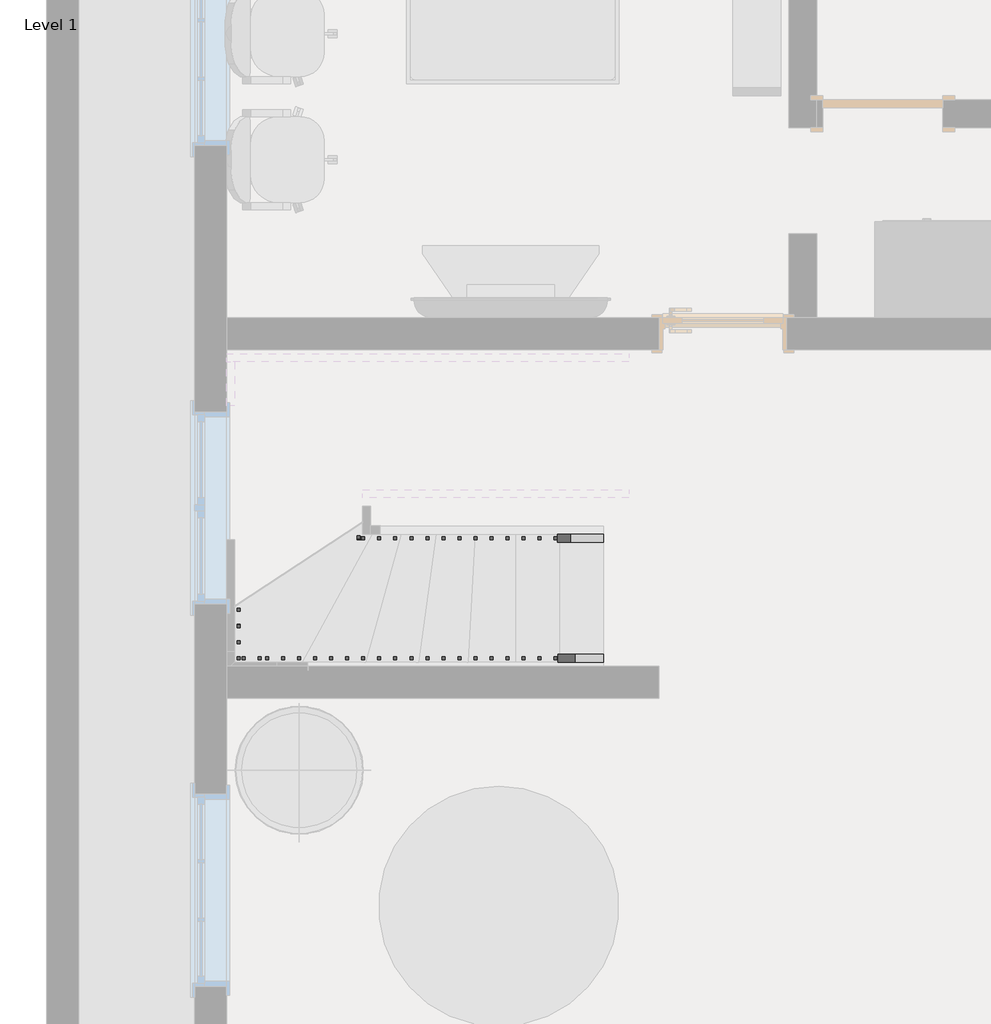
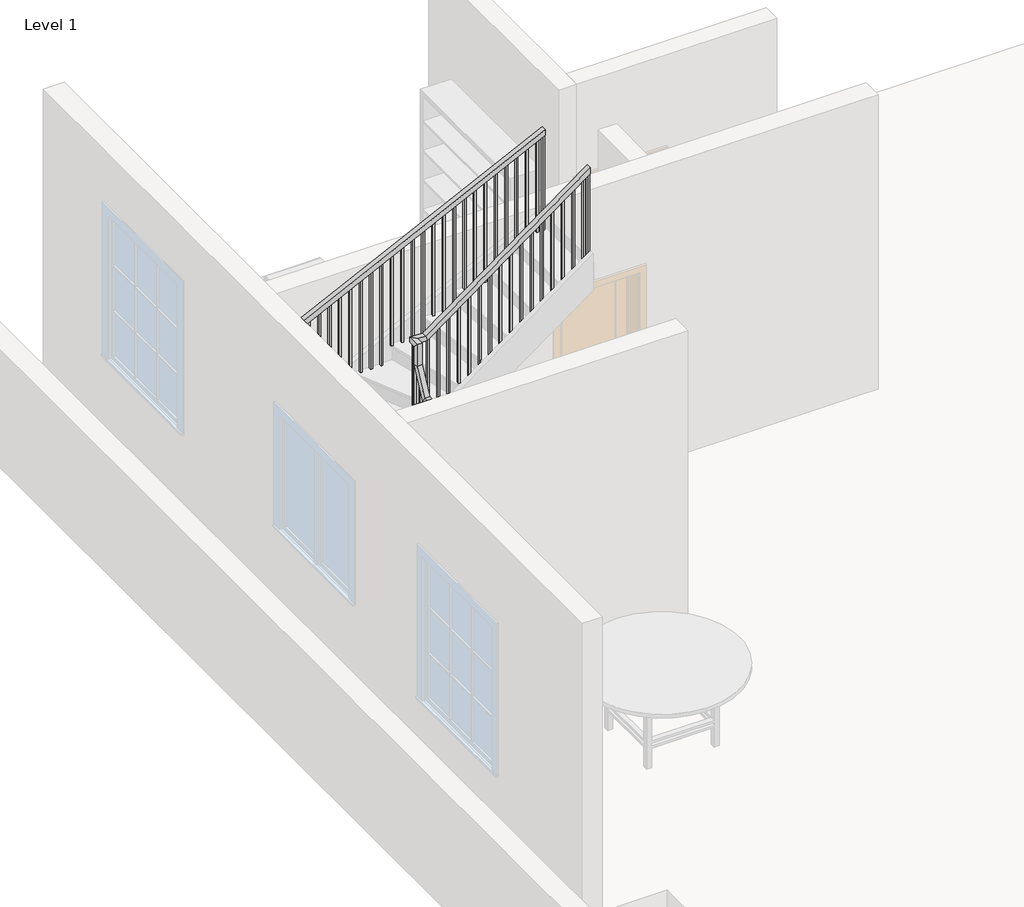
# One storey, part 2 of 3: 2 railings.
"""IFC4 building model written with IfcOpenShell, lengths in millimetres."""

from ifc_helpers import new_model, si_unit, frame, origin, place, context, project, spatial, polyline, outline, extrude, faceted_brep, element, save

model = new_model("IFC4")

# Units and contexts
model_context = context("Model", 3, world=origin())
ifc_project = project(units=[si_unit("LENGTHUNIT", "METRE", prefix="MILLI")], contexts=[model_context])

# Site, building, storey
site = spatial("IfcSite", under=ifc_project)
building = spatial("IfcBuilding", under=site)
storey = spatial("IfcBuildingStorey", under=building, Name="Level 1", Elevation=0.0)

# Railings
placement = place(None, origin())
element("IfcRailing", 1, ObjectType="Handrail - Rectangular", at=placement, inside=storey, context=model_context, shape_type="SolidModel", body=[
    faceted_brep([(-12253.9414615, 8938.3162111, 1054.0374735), (-12253.9414615, 8938.3162111, 991.6664218), (-12253.9414615, 8989.1162111, 991.6664218), (-12253.9414615, 8989.1162111, 1054.0374735), (-13705.4731534, 8938.3162111, 2088.0288176), (-13756.2731534, 8938.3162111, 2061.8448919), (-13756.2731534, 8989.1162111, 2061.8448919), (-13705.4731534, 8989.1162111, 2088.0288176), (-13705.4731534, 8938.3162111, 2341.1218659), (-13756.2731534, 8938.3162111, 2290.3218659), (-13756.2731534, 8989.1162111, 2290.3218659), (-13705.4731534, 8989.1162111, 2341.1218659), (-13832.4731534, 8938.3162111, 2341.1218659), (-13832.4731534, 8938.3162111, 2290.3218659), (-13781.6731534, 8989.1162111, 2290.3218659), (-13781.6731534, 8989.1162111, 2341.1218659), (-13832.4731534, 9065.3162111, 2341.1218659), (-13832.4731534, 9096.7018628, 2290.3218659), (-13781.6731534, 9096.7018628, 2290.3218659), (-13781.6731534, 9065.3162111, 2341.1218659), (-13832.4731534, 9192.3162111, 2594.9324677), (-13832.4731534, 9243.1162111, 2582.9322113), (-13781.6731534, 9243.1162111, 2582.9322113), (-13781.6731534, 9192.3162111, 2594.9324677), (-13832.4731534, 9192.3162111, 2819.759768), (-13832.4731534, 9243.1162111, 2768.959768), (-13781.6731534, 9243.1162111, 2768.959768), (-13781.6731534, 9192.3162111, 2819.759768), (-13832.4731534, 9319.3162111, 2819.759768), (-13832.4731534, 9319.3162111, 2768.959768), (-13781.6731534, 9268.5162111, 2768.959768), (-13781.6731534, 9268.5162111, 2819.759768), (-13705.4731534, 9319.3162111, 2819.759768), (-13688.9113924, 9319.3162111, 2768.959768), (-13688.9113924, 9268.5162111, 2768.959768), (-13705.4731534, 9268.5162111, 2819.759768), (-12092.016007, 9319.3162111, 3996.9124676), (-12092.016007, 9268.5162111, 3996.9124676), (-12092.016007, 9268.5162111, 3934.0292699), (-12092.016007, 9319.3162111, 3934.0292699)], [[[0, 1, 2, 3]], [[1, 0, 4, 5]], [[2, 1, 5, 6]], [[3, 2, 6, 7]], [[0, 3, 7, 4]], [[5, 4, 8, 9]], [[6, 5, 9, 10]], [[7, 6, 10, 11]], [[4, 7, 11, 8]], [[9, 8, 12, 13]], [[10, 9, 13, 14]], [[11, 10, 14, 15]], [[8, 11, 15, 12]], [[13, 12, 16, 17]], [[14, 13, 17, 18]], [[15, 14, 18, 19]], [[12, 15, 19, 16]], [[17, 16, 20, 21]], [[18, 17, 21, 22]], [[19, 18, 22, 23]], [[16, 19, 23, 20]], [[21, 20, 24, 25]], [[22, 21, 25, 26]], [[23, 22, 26, 27]], [[20, 23, 27, 24]], [[25, 24, 28, 29]], [[26, 25, 29, 30]], [[27, 26, 30, 31]], [[24, 27, 31, 28]], [[29, 28, 32, 33]], [[30, 29, 33, 34]], [[31, 30, 34, 35]], [[28, 31, 35, 32]], [[36, 37, 38, 39]], [[33, 32, 36, 39]], [[34, 33, 39, 38]], [[35, 34, 38, 37]], [[32, 35, 37, 36]]]),
    extrude(outline(polyline([(3901.8855094, -12136.0736558), (3887.986932, -12155.1236558), (2878.6666667, -12155.1236558), (2878.6666667, -12136.0736558), (3901.8855094, -12136.0736558)])), frame((0.0, 9284.3912111, 0.0), z_axis=(0.0, 1.0, 0.0), x_axis=(0.0, 0.0, 1.0)), (0.0, 0.0, 1.0), 19.05),
    extrude(outline(polyline([(3827.7597636, -12237.6736558), (3813.8611863, -12256.7236558), (2878.6666667, -12256.7236558), (2878.6666667, -12237.6736558), (3827.7597636, -12237.6736558)])), frame((0.0, 9284.3912111, 0.0), z_axis=(0.0, 1.0, 0.0), x_axis=(0.0, 0.0, 1.0)), (0.0, 0.0, 1.0), 19.05),
    extrude(outline(polyline([(3753.6340178, -12339.2736558), (3739.7354405, -12358.3236558), (2878.6666667, -12358.3236558), (2878.6666667, -12339.2736558), (3753.6340178, -12339.2736558)])), frame((0.0, 9284.3912111, 0.0), z_axis=(0.0, 1.0, 0.0), x_axis=(0.0, 0.0, 1.0)), (0.0, 0.0, 1.0), 19.05),
    extrude(outline(polyline([(3679.508272, -12440.8736558), (3665.6096947, -12459.9236558), (2709.3333333, -12459.9236558), (2709.3333333, -12440.8736558), (3679.508272, -12440.8736558)])), frame((0.0, 9284.3912111, 0.0), z_axis=(0.0, 1.0, 0.0), x_axis=(0.0, 0.0, 1.0)), (0.0, 0.0, 1.0), 19.05),
    extrude(outline(polyline([(3605.3825262, -12542.4736558), (3591.4839489, -12561.5236558), (2709.3333333, -12561.5236558), (2709.3333333, -12542.4736558), (3605.3825262, -12542.4736558)])), frame((0.0, 9284.3912111, 0.0), z_axis=(0.0, 1.0, 0.0), x_axis=(0.0, 0.0, 1.0)), (0.0, 0.0, 1.0), 19.05),
    extrude(outline(polyline([(3531.2567804, -12644.0736558), (3517.3582031, -12663.1236558), (2540.0, -12663.1236558), (2540.0, -12644.0736558), (3531.2567804, -12644.0736558)])), frame((0.0, 9284.3912111, 0.0), z_axis=(0.0, 1.0, 0.0), x_axis=(0.0, 0.0, 1.0)), (0.0, 0.0, 1.0), 19.05),
    extrude(outline(polyline([(3457.1310346, -12745.6736558), (3443.2324573, -12764.7236558), (2540.0, -12764.7236558), (2540.0, -12745.6736558), (3457.1310346, -12745.6736558)])), frame((0.0, 9284.3912111, 0.0), z_axis=(0.0, 1.0, 0.0), x_axis=(0.0, 0.0, 1.0)), (0.0, 0.0, 1.0), 19.05),
    extrude(outline(polyline([(3383.0052889, -12847.2736558), (3369.1067115, -12866.3236558), (2540.0, -12866.3236558), (2540.0, -12847.2736558), (3383.0052889, -12847.2736558)])), frame((0.0, 9284.3912111, 0.0), z_axis=(0.0, 1.0, 0.0), x_axis=(0.0, 0.0, 1.0)), (0.0, 0.0, 1.0), 19.05),
    extrude(outline(polyline([(3308.8795431, -12948.8736558), (3294.9809657, -12967.9236558), (2370.6666667, -12967.9236558), (2370.6666667, -12948.8736558), (3308.8795431, -12948.8736558)])), frame((0.0, 9284.3912111, 0.0), z_axis=(0.0, 1.0, 0.0), x_axis=(0.0, 0.0, 1.0)), (0.0, 0.0, 1.0), 19.05),
    extrude(outline(polyline([(3234.7537973, -13050.4736558), (3220.8552199, -13069.5236558), (2370.6666667, -13069.5236558), (2370.6666667, -13050.4736558), (3234.7537973, -13050.4736558)])), frame((0.0, 9284.3912111, 0.0), z_axis=(0.0, 1.0, 0.0), x_axis=(0.0, 0.0, 1.0)), (0.0, 0.0, 1.0), 19.05),
    extrude(outline(polyline([(3160.6280515, -13152.0736558), (3146.7294741, -13171.1236558), (2201.3333333, -13171.1236558), (2201.3333333, -13152.0736558), (3160.6280515, -13152.0736558)])), frame((0.0, 9284.3912111, 0.0), z_axis=(0.0, 1.0, 0.0), x_axis=(0.0, 0.0, 1.0)), (0.0, 0.0, 1.0), 19.05),
    extrude(outline(polyline([(3086.5023057, -13253.6736558), (3072.6037284, -13272.7236558), (2201.3333333, -13272.7236558), (2201.3333333, -13253.6736558), (3086.5023057, -13253.6736558)])), frame((0.0, 9284.3912111, 0.0), z_axis=(0.0, 1.0, 0.0), x_axis=(0.0, 0.0, 1.0)), (0.0, 0.0, 1.0), 19.05),
    extrude(outline(polyline([(3012.3765599, -13355.2736558), (2998.4779826, -13374.3236558), (2201.3333333, -13374.3236558), (2201.3333333, -13355.2736558), (3012.3765599, -13355.2736558)])), frame((0.0, 9284.3912111, 0.0), z_axis=(0.0, 1.0, 0.0), x_axis=(0.0, 0.0, 1.0)), (0.0, 0.0, 1.0), 19.05),
    extrude(outline(polyline([(2938.2508141, -13456.8736558), (2924.3522368, -13475.9236558), (2032.0, -13475.9236558), (2032.0, -13456.8736558), (2938.2508141, -13456.8736558)])), frame((0.0, 9284.3912111, 0.0), z_axis=(0.0, 1.0, 0.0), x_axis=(0.0, 0.0, 1.0)), (0.0, 0.0, 1.0), 19.05),
    extrude(outline(polyline([(2864.1250683, -13558.4736558), (2850.226491, -13577.5236558), (2032.0, -13577.5236558), (2032.0, -13558.4736558), (2864.1250683, -13558.4736558)])), frame((0.0, 9284.3912111, 0.0), z_axis=(0.0, 1.0, 0.0), x_axis=(0.0, 0.0, 1.0)), (0.0, 0.0, 1.0), 19.05),
    extrude(outline(polyline([(2789.9993225, -13660.0736558), (2776.1007452, -13679.1236558), (1862.6666667, -13679.1236558), (1862.6666667, -13660.0736558), (2789.9993225, -13660.0736558)])), frame((0.0, 9284.3912111, 0.0), z_axis=(0.0, 1.0, 0.0), x_axis=(0.0, 0.0, 1.0)), (0.0, 0.0, 1.0), 19.05),
    extrude(outline(polyline([(-13797.5481534, 9264.5777982), (-13816.5981534, 9264.5777982), (-13816.5981534, 9283.6277982), (-13797.5481534, 9283.6277982), (-13797.5481534, 9264.5777982)])), frame((0.0, 0.0, 1693.3333333), z_axis=(0.0, 0.0, 1.0), x_axis=(1.0, 0.0, 0.0)), (0.0, 0.0, 1.0), 1075.6264347),
    extrude(outline(polyline([(9162.9777982, 2422.7748977), (9182.0277982, 2460.846488), (9182.0277982, 1524.0), (9162.9777982, 1524.0), (9162.9777982, 2422.7748977)])), frame((-13816.5981534, 0.0, 0.0), z_axis=(1.0, 0.0, 0.0), x_axis=(0.0, 1.0, 0.0)), (0.0, 0.0, 1.0), 19.05),
    extrude(outline(polyline([(9061.3777982, 2219.7264162), (9080.4277982, 2257.7980065), (9080.4277982, 1354.6666667), (9061.3777982, 1354.6666667), (9061.3777982, 2219.7264162)])), frame((-13816.5981534, 0.0, 0.0), z_axis=(1.0, 0.0, 0.0), x_axis=(0.0, 1.0, 0.0)), (0.0, 0.0, 1.0), 19.05),
    extrude(outline(polyline([(-13768.4164615, 8973.2412111), (-13768.4164615, 8954.1912111), (-13787.4664615, 8954.1912111), (-13787.4664615, 8973.2412111), (-13768.4164615, 8973.2412111)])), frame((0.0, 0.0, 1185.3333333), z_axis=(0.0, 0.0, 1.0), x_axis=(1.0, 0.0, 0.0)), (0.0, 0.0, 1.0), 1104.9885325),
    extrude(outline(polyline([(1998.1208647, -13666.8164615), (2011.691037, -13685.8664615), (1016.0, -13685.8664615), (1016.0, -13666.8164615), (1998.1208647, -13666.8164615)])), frame((0.0, 8954.1912111, 0.0), z_axis=(0.0, 1.0, 0.0), x_axis=(0.0, 0.0, 1.0)), (0.0, 0.0, 1.0), 19.05),
    extrude(outline(polyline([(1925.7466126, -13565.2164615), (1939.3167849, -13584.2664615), (1016.0, -13584.2664615), (1016.0, -13565.2164615), (1925.7466126, -13565.2164615)])), frame((0.0, 8954.1912111, 0.0), z_axis=(0.0, 1.0, 0.0), x_axis=(0.0, 0.0, 1.0)), (0.0, 0.0, 1.0), 19.05),
    extrude(outline(polyline([(1853.3723605, -13463.6164615), (1866.9425328, -13482.6664615), (846.6666667, -13482.6664615), (846.6666667, -13463.6164615), (1853.3723605, -13463.6164615)])), frame((0.0, 8954.1912111, 0.0), z_axis=(0.0, 1.0, 0.0), x_axis=(0.0, 0.0, 1.0)), (0.0, 0.0, 1.0), 19.05),
    extrude(outline(polyline([(1780.9981085, -13362.0164615), (1794.5682807, -13381.0664615), (846.6666667, -13381.0664615), (846.6666667, -13362.0164615), (1780.9981085, -13362.0164615)])), frame((0.0, 8954.1912111, 0.0), z_axis=(0.0, 1.0, 0.0), x_axis=(0.0, 0.0, 1.0)), (0.0, 0.0, 1.0), 19.05),
    extrude(outline(polyline([(1708.6238564, -13260.4164615), (1722.1940286, -13279.4664615), (677.3333333, -13279.4664615), (677.3333333, -13260.4164615), (1708.6238564, -13260.4164615)])), frame((0.0, 8954.1912111, 0.0), z_axis=(0.0, 1.0, 0.0), x_axis=(0.0, 0.0, 1.0)), (0.0, 0.0, 1.0), 19.05),
    extrude(outline(polyline([(1636.2496043, -13158.8164615), (1649.8197766, -13177.8664615), (677.3333333, -13177.8664615), (677.3333333, -13158.8164615), (1636.2496043, -13158.8164615)])), frame((0.0, 8954.1912111, 0.0), z_axis=(0.0, 1.0, 0.0), x_axis=(0.0, 0.0, 1.0)), (0.0, 0.0, 1.0), 19.05),
    extrude(outline(polyline([(1563.8753522, -13057.2164615), (1577.4455245, -13076.2664615), (508.0, -13076.2664615), (508.0, -13057.2164615), (1563.8753522, -13057.2164615)])), frame((0.0, 8954.1912111, 0.0), z_axis=(0.0, 1.0, 0.0), x_axis=(0.0, 0.0, 1.0)), (0.0, 0.0, 1.0), 19.05),
    extrude(outline(polyline([(1491.5011002, -12955.6164615), (1505.0712724, -12974.6664615), (508.0, -12974.6664615), (508.0, -12955.6164615), (1491.5011002, -12955.6164615)])), frame((0.0, 8954.1912111, 0.0), z_axis=(0.0, 1.0, 0.0), x_axis=(0.0, 0.0, 1.0)), (0.0, 0.0, 1.0), 19.05),
    extrude(outline(polyline([(1419.1268481, -12854.0164615), (1432.6970203, -12873.0664615), (508.0, -12873.0664615), (508.0, -12854.0164615), (1419.1268481, -12854.0164615)])), frame((0.0, 8954.1912111, 0.0), z_axis=(0.0, 1.0, 0.0), x_axis=(0.0, 0.0, 1.0)), (0.0, 0.0, 1.0), 19.05),
    extrude(outline(polyline([(1346.752596, -12752.4164615), (1360.3227683, -12771.4664615), (338.6666667, -12771.4664615), (338.6666667, -12752.4164615), (1346.752596, -12752.4164615)])), frame((0.0, 8954.1912111, 0.0), z_axis=(0.0, 1.0, 0.0), x_axis=(0.0, 0.0, 1.0)), (0.0, 0.0, 1.0), 19.05),
    extrude(outline(polyline([(1274.3783439, -12650.8164615), (1287.9485162, -12669.8664615), (338.6666667, -12669.8664615), (338.6666667, -12650.8164615), (1274.3783439, -12650.8164615)])), frame((0.0, 8954.1912111, 0.0), z_axis=(0.0, 1.0, 0.0), x_axis=(0.0, 0.0, 1.0)), (0.0, 0.0, 1.0), 19.05),
    extrude(outline(polyline([(1202.0040918, -12549.2164615), (1215.5742641, -12568.2664615), (338.6666667, -12568.2664615), (338.6666667, -12549.2164615), (1202.0040918, -12549.2164615)])), frame((0.0, 8954.1912111, 0.0), z_axis=(0.0, 1.0, 0.0), x_axis=(0.0, 0.0, 1.0)), (0.0, 0.0, 1.0), 19.05),
    extrude(outline(polyline([(1129.6298398, -12447.6164615), (1143.200012, -12466.6664615), (169.3333333, -12466.6664615), (169.3333333, -12447.6164615), (1129.6298398, -12447.6164615)])), frame((0.0, 8954.1912111, 0.0), z_axis=(0.0, 1.0, 0.0), x_axis=(0.0, 0.0, 1.0)), (0.0, 0.0, 1.0), 19.05),
    extrude(outline(polyline([(1057.2555877, -12346.0164615), (1070.82576, -12365.0664615), (169.3333333, -12365.0664615), (169.3333333, -12346.0164615), (1057.2555877, -12346.0164615)])), frame((0.0, 8954.1912111, 0.0), z_axis=(0.0, 1.0, 0.0), x_axis=(0.0, 0.0, 1.0)), (0.0, 0.0, 1.0), 19.05),
    extrude(outline(polyline([(-13780.7236558, 9284.3912111), (-13780.7236558, 9303.4412111), (-13761.6736558, 9303.4412111), (-13761.6736558, 9284.3912111), (-13780.7236558, 9284.3912111)])), frame((0.0, 0.0, 1862.6666667), z_axis=(0.0, 0.0, 1.0), x_axis=(1.0, 0.0, 0.0)), (0.0, 0.0, 1.0), 906.2931014),
    extrude(outline(polyline([(-13797.5481534, 9284.3912111), (-13816.5981534, 9284.3912111), (-13816.5981534, 9303.4412111), (-13797.5481534, 9303.4412111), (-13797.5481534, 9284.3912111)])), frame((0.0, 0.0, 1693.3333333), z_axis=(0.0, 0.0, 1.0), x_axis=(1.0, 0.0, 0.0)), (0.0, 0.0, 1.0), 1075.6264347),
    extrude(outline(polyline([(-13797.5481534, 9271.2947138), (-13816.5981534, 9271.2947138), (-13816.5981534, 9290.3447138), (-13797.5481534, 9290.3447138), (-13797.5481534, 9271.2947138)])), frame((0.0, 0.0, 1693.3333333), z_axis=(0.0, 0.0, 1.0), x_axis=(1.0, 0.0, 0.0)), (0.0, 0.0, 1.0), 1075.6264347),
    extrude(outline(polyline([(-13797.5481534, 8959.7777982), (-13816.5981534, 8959.7777982), (-13816.5981534, 8978.8277982), (-13797.5481534, 8978.8277982), (-13797.5481534, 8959.7777982)])), frame((0.0, 0.0, 1185.3333333), z_axis=(0.0, 0.0, 1.0), x_axis=(1.0, 0.0, 0.0)), (0.0, 0.0, 1.0), 1104.9885325),
    extrude(outline(polyline([(-13797.5481534, 8973.2412111), (-13797.5481534, 8954.1912111), (-13816.5981534, 8954.1912111), (-13816.5981534, 8973.2412111), (-13797.5481534, 8973.2412111)])), frame((0.0, 0.0, 1185.3333333), z_axis=(0.0, 0.0, 1.0), x_axis=(1.0, 0.0, 0.0)), (0.0, 0.0, 1.0), 1104.9885325),
    extrude(outline(polyline([(-13781.8747892, 8973.2412111), (-13781.8747892, 8954.1912111), (-13800.9247892, 8954.1912111), (-13800.9247892, 8973.2412111), (-13781.8747892, 8973.2412111)])), frame((0.0, 0.0, 1185.3333333), z_axis=(0.0, 0.0, 1.0), x_axis=(1.0, 0.0, 0.0)), (0.0, 0.0, 1.0), 1104.9885325),
    extrude(outline(polyline([(3934.0292699, -12092.016007), (3920.1306926, -12111.066007), (2878.6666667, -12111.066007), (2878.6666667, -12092.016007), (3934.0292699, -12092.016007)])), frame((0.0, 9284.3912111, 0.0), z_axis=(0.0, 1.0, 0.0), x_axis=(0.0, 0.0, 1.0)), (0.0, 0.0, 1.0), 19.05),
    extrude(outline(polyline([(991.6664218, -12253.9414615), (1005.236594, -12272.9914615), (169.3333333, -12272.9914615), (169.3333333, -12253.9414615), (991.6664218, -12253.9414615)])), frame((0.0, 8954.1912111, 0.0), z_axis=(0.0, 1.0, 0.0), x_axis=(0.0, 0.0, 1.0)), (0.0, 0.0, 1.0), 19.05),
])
element("IfcRailing", 2, ObjectType="Handrail - Rectangular", at=placement, inside=storey, context=model_context, shape_type="SolidModel", body=[
    faceted_brep([(-12253.9414615, 8176.3162111, 1108.1974031), (-12253.9414615, 8176.3162111, 1050.9747805), (-12253.9414615, 8227.1162111, 1050.9747805), (-12253.9414615, 8227.1162111, 1108.1974031), (-14435.851857, 8176.3162111, 2239.520782), (-14448.2387549, 8176.3162111, 2188.720782), (-14448.2387549, 8227.1162111, 2188.720782), (-14435.851857, 8227.1162111, 2239.520782), (-14594.4731534, 8176.3162111, 2239.520782), (-14594.4731534, 8176.3162111, 2188.720782), (-14543.6731534, 8227.1162111, 2188.720782), (-14543.6731534, 8227.1162111, 2239.520782), (-14594.4731534, 8407.7273211, 2239.520782), (-14594.4731534, 8416.0171351, 2188.720782), (-14543.6731534, 8416.0171351, 2188.720782), (-14543.6731534, 8407.7273211, 2239.520782), (-14594.4731534, 9947.9383629, 2755.9527245), (-14594.4731534, 9956.2281769, 2705.1527245), (-14543.6731534, 9956.2281769, 2705.1527245), (-14543.6731534, 9947.9383629, 2755.9527245), (-14594.4731534, 10081.3162111, 2755.9527245), (-14594.4731534, 10081.3162111, 2705.1527245), (-14543.6731534, 10030.5162111, 2705.1527245), (-14543.6731534, 10030.5162111, 2755.9527245), (-14494.942349, 10081.3162111, 2755.9527245), (-14483.1999894, 10081.3162111, 2705.1527245), (-14483.1999894, 10030.5162111, 2705.1527245), (-14494.942349, 10030.5162111, 2755.9527245), (-12092.016007, 10081.3162111, 3929.523479), (-12092.016007, 10030.5162111, 3929.523479), (-12092.016007, 10030.5162111, 3872.9886008), (-12092.016007, 10081.3162111, 3872.9886008)], [[[0, 1, 2, 3]], [[1, 0, 4, 5]], [[2, 1, 5, 6]], [[3, 2, 6, 7]], [[0, 3, 7, 4]], [[5, 4, 8, 9]], [[6, 5, 9, 10]], [[7, 6, 10, 11]], [[4, 7, 11, 8]], [[9, 8, 12, 13]], [[10, 9, 13, 14]], [[11, 10, 14, 15]], [[8, 11, 15, 12]], [[13, 12, 16, 17]], [[14, 13, 17, 18]], [[15, 14, 18, 19]], [[12, 15, 19, 16]], [[17, 16, 20, 21]], [[18, 17, 21, 22]], [[19, 18, 22, 23]], [[16, 19, 23, 20]], [[21, 20, 24, 25]], [[22, 21, 25, 26]], [[23, 22, 26, 27]], [[20, 23, 27, 24]], [[28, 29, 30, 31]], [[25, 24, 28, 31]], [[26, 25, 31, 30]], [[27, 26, 30, 29]], [[24, 27, 29, 28]]]),
    extrude(outline(polyline([(3836.0410669, -12167.667349), (2878.6666667, -12167.667349), (2878.6666667, -12148.617349), (3845.3449404, -12148.617349), (3836.0410669, -12167.667349)])), frame((0.0, 10046.3912111, 0.0), z_axis=(0.0, 1.0, 0.0), x_axis=(0.0, 0.0, 1.0)), (0.0, 0.0, 1.0), 19.05),
    extrude(outline(polyline([(3786.4204079, -12269.267349), (2878.6666667, -12269.267349), (2878.6666667, -12250.217349), (3795.7242814, -12250.217349), (3786.4204079, -12269.267349)])), frame((0.0, 10046.3912111, 0.0), z_axis=(0.0, 1.0, 0.0), x_axis=(0.0, 0.0, 1.0)), (0.0, 0.0, 1.0), 19.05),
    extrude(outline(polyline([(3736.7997488, -12370.867349), (2878.6666667, -12370.867349), (2878.6666667, -12351.817349), (3746.1036224, -12351.817349), (3736.7997488, -12370.867349)])), frame((0.0, 10046.3912111, 0.0), z_axis=(0.0, 1.0, 0.0), x_axis=(0.0, 0.0, 1.0)), (0.0, 0.0, 1.0), 19.05),
    extrude(outline(polyline([(3687.1790898, -12472.467349), (2709.3333333, -12472.467349), (2709.3333333, -12453.417349), (3696.4829634, -12453.417349), (3687.1790898, -12472.467349)])), frame((0.0, 10046.3912111, 0.0), z_axis=(0.0, 1.0, 0.0), x_axis=(0.0, 0.0, 1.0)), (0.0, 0.0, 1.0), 19.05),
    extrude(outline(polyline([(3637.5584308, -12574.067349), (2709.3333333, -12574.067349), (2709.3333333, -12555.017349), (3646.8623044, -12555.017349), (3637.5584308, -12574.067349)])), frame((0.0, 10046.3912111, 0.0), z_axis=(0.0, 1.0, 0.0), x_axis=(0.0, 0.0, 1.0)), (0.0, 0.0, 1.0), 19.05),
    extrude(outline(polyline([(3587.9377718, -12675.667349), (2540.0, -12675.667349), (2540.0, -12656.617349), (3597.2416454, -12656.617349), (3587.9377718, -12675.667349)])), frame((0.0, 10046.3912111, 0.0), z_axis=(0.0, 1.0, 0.0), x_axis=(0.0, 0.0, 1.0)), (0.0, 0.0, 1.0), 19.05),
    extrude(outline(polyline([(3538.3171128, -12777.267349), (2540.0, -12777.267349), (2540.0, -12758.217349), (3547.6209864, -12758.217349), (3538.3171128, -12777.267349)])), frame((0.0, 10046.3912111, 0.0), z_axis=(0.0, 1.0, 0.0), x_axis=(0.0, 0.0, 1.0)), (0.0, 0.0, 1.0), 19.05),
    extrude(outline(polyline([(3488.6964538, -12878.867349), (2540.0, -12878.867349), (2540.0, -12859.817349), (3498.0003273, -12859.817349), (3488.6964538, -12878.867349)])), frame((0.0, 10046.3912111, 0.0), z_axis=(0.0, 1.0, 0.0), x_axis=(0.0, 0.0, 1.0)), (0.0, 0.0, 1.0), 19.05),
    extrude(outline(polyline([(3439.0757948, -12980.467349), (2370.6666667, -12980.467349), (2370.6666667, -12961.417349), (3448.3796683, -12961.417349), (3439.0757948, -12980.467349)])), frame((0.0, 10046.3912111, 0.0), z_axis=(0.0, 1.0, 0.0), x_axis=(0.0, 0.0, 1.0)), (0.0, 0.0, 1.0), 19.05),
    extrude(outline(polyline([(3389.4551357, -13082.067349), (2370.6666667, -13082.067349), (2370.6666667, -13063.017349), (3398.7590093, -13063.017349), (3389.4551357, -13082.067349)])), frame((0.0, 10046.3912111, 0.0), z_axis=(0.0, 1.0, 0.0), x_axis=(0.0, 0.0, 1.0)), (0.0, 0.0, 1.0), 19.05),
    extrude(outline(polyline([(3339.8344767, -13183.667349), (2370.6666667, -13183.667349), (2370.6666667, -13164.617349), (3349.1383503, -13164.617349), (3339.8344767, -13183.667349)])), frame((0.0, 10046.3912111, 0.0), z_axis=(0.0, 1.0, 0.0), x_axis=(0.0, 0.0, 1.0)), (0.0, 0.0, 1.0), 19.05),
    extrude(outline(polyline([(3290.2138177, -13285.267349), (2201.3333333, -13285.267349), (2201.3333333, -13266.217349), (3299.5176913, -13266.217349), (3290.2138177, -13285.267349)])), frame((0.0, 10046.3912111, 0.0), z_axis=(0.0, 1.0, 0.0), x_axis=(0.0, 0.0, 1.0)), (0.0, 0.0, 1.0), 19.05),
    extrude(outline(polyline([(3240.5931587, -13386.867349), (2201.3333333, -13386.867349), (2201.3333333, -13367.817349), (3249.8970323, -13367.817349), (3240.5931587, -13386.867349)])), frame((0.0, 10046.3912111, 0.0), z_axis=(0.0, 1.0, 0.0), x_axis=(0.0, 0.0, 1.0)), (0.0, 0.0, 1.0), 19.05),
    extrude(outline(polyline([(3190.9724997, -13488.467349), (2201.3333333, -13488.467349), (2201.3333333, -13469.417349), (3200.2763733, -13469.417349), (3190.9724997, -13488.467349)])), frame((0.0, 10046.3912111, 0.0), z_axis=(0.0, 1.0, 0.0), x_axis=(0.0, 0.0, 1.0)), (0.0, 0.0, 1.0), 19.05),
    extrude(outline(polyline([(3141.3518407, -13590.067349), (2201.3333333, -13590.067349), (2201.3333333, -13571.017349), (3150.6557142, -13571.017349), (3141.3518407, -13590.067349)])), frame((0.0, 10046.3912111, 0.0), z_axis=(0.0, 1.0, 0.0), x_axis=(0.0, 0.0, 1.0)), (0.0, 0.0, 1.0), 19.05),
    extrude(outline(polyline([(3091.7311817, -13691.667349), (2032.0, -13691.667349), (2032.0, -13672.617349), (3101.0350552, -13672.617349), (3091.7311817, -13691.667349)])), frame((0.0, 10046.3912111, 0.0), z_axis=(0.0, 1.0, 0.0), x_axis=(0.0, 0.0, 1.0)), (0.0, 0.0, 1.0), 19.05),
    extrude(outline(polyline([(3042.1105226, -13793.267349), (2032.0, -13793.267349), (2032.0, -13774.217349), (3051.4143962, -13774.217349), (3042.1105226, -13793.267349)])), frame((0.0, 10046.3912111, 0.0), z_axis=(0.0, 1.0, 0.0), x_axis=(0.0, 0.0, 1.0)), (0.0, 0.0, 1.0), 19.05),
    extrude(outline(polyline([(2992.4898636, -13894.867349), (2032.0, -13894.867349), (2032.0, -13875.817349), (3001.7937372, -13875.817349), (2992.4898636, -13894.867349)])), frame((0.0, 10046.3912111, 0.0), z_axis=(0.0, 1.0, 0.0), x_axis=(0.0, 0.0, 1.0)), (0.0, 0.0, 1.0), 19.05),
    extrude(outline(polyline([(2942.8692046, -13996.467349), (1862.6666667, -13996.467349), (1862.6666667, -13977.417349), (2952.1730782, -13977.417349), (2942.8692046, -13996.467349)])), frame((0.0, 10046.3912111, 0.0), z_axis=(0.0, 1.0, 0.0), x_axis=(0.0, 0.0, 1.0)), (0.0, 0.0, 1.0), 19.05),
    extrude(outline(polyline([(2893.2485456, -14098.067349), (1862.6666667, -14098.067349), (1862.6666667, -14079.017349), (2902.5524192, -14079.017349), (2893.2485456, -14098.067349)])), frame((0.0, 10046.3912111, 0.0), z_axis=(0.0, 1.0, 0.0), x_axis=(0.0, 0.0, 1.0)), (0.0, 0.0, 1.0), 19.05),
    extrude(outline(polyline([(2843.6278866, -14199.667349), (1862.6666667, -14199.667349), (1862.6666667, -14180.617349), (2852.9317602, -14180.617349), (2843.6278866, -14199.667349)])), frame((0.0, 10046.3912111, 0.0), z_axis=(0.0, 1.0, 0.0), x_axis=(0.0, 0.0, 1.0)), (0.0, 0.0, 1.0), 19.05),
    extrude(outline(polyline([(2794.0072276, -14301.267349), (1862.6666667, -14301.267349), (1862.6666667, -14282.217349), (2803.3111011, -14282.217349), (2794.0072276, -14301.267349)])), frame((0.0, 10046.3912111, 0.0), z_axis=(0.0, 1.0, 0.0), x_axis=(0.0, 0.0, 1.0)), (0.0, 0.0, 1.0), 19.05),
    extrude(outline(polyline([(2744.3865686, -14402.867349), (1862.6666667, -14402.867349), (1862.6666667, -14383.817349), (2753.6904421, -14383.817349), (2744.3865686, -14402.867349)])), frame((0.0, 10046.3912111, 0.0), z_axis=(0.0, 1.0, 0.0), x_axis=(0.0, 0.0, 1.0)), (0.0, 0.0, 1.0), 19.05),
    extrude(outline(polyline([(-14578.5981534, 10040.0133629), (-14578.5981534, 10059.0633629), (-14559.5481534, 10059.0633629), (-14559.5481534, 10040.0133629), (-14578.5981534, 10040.0133629)])), frame((0.0, 0.0, 1693.3333333), z_axis=(0.0, 0.0, 1.0), x_axis=(1.0, 0.0, 0.0)), (0.0, 0.0, 1.0), 1011.8193912),
    extrude(outline(polyline([(9941.2523211, 2700.131328), (9941.2523211, 1693.3333333), (9922.2023211, 1693.3333333), (9922.2023211, 2693.7438732), (9941.2523211, 2700.131328)])), frame((-14578.5981534, 0.0, 0.0), z_axis=(1.0, 0.0, 0.0), x_axis=(0.0, 1.0, 0.0)), (0.0, 0.0, 1.0), 19.05),
    extrude(outline(polyline([(9839.6523211, 2666.0649021), (9839.6523211, 1693.3333333), (9820.6023211, 1693.3333333), (9820.6023211, 2659.6774473), (9839.6523211, 2666.0649021)])), frame((-14578.5981534, 0.0, 0.0), z_axis=(1.0, 0.0, 0.0), x_axis=(0.0, 1.0, 0.0)), (0.0, 0.0, 1.0), 19.05),
    extrude(outline(polyline([(9738.0523211, 2631.9984762), (9738.0523211, 1693.3333333), (9719.0023211, 1693.3333333), (9719.0023211, 2625.6110213), (9738.0523211, 2631.9984762)])), frame((-14578.5981534, 0.0, 0.0), z_axis=(1.0, 0.0, 0.0), x_axis=(0.0, 1.0, 0.0)), (0.0, 0.0, 1.0), 19.05),
    extrude(outline(polyline([(9636.4523211, 2597.9320503), (9636.4523211, 1693.3333333), (9617.4023211, 1693.3333333), (9617.4023211, 2591.5445954), (9636.4523211, 2597.9320503)])), frame((-14578.5981534, 0.0, 0.0), z_axis=(1.0, 0.0, 0.0), x_axis=(0.0, 1.0, 0.0)), (0.0, 0.0, 1.0), 19.05),
    extrude(outline(polyline([(9534.8523211, 2563.8656244), (9534.8523211, 1693.3333333), (9515.8023211, 1693.3333333), (9515.8023211, 2557.4781695), (9534.8523211, 2563.8656244)])), frame((-14578.5981534, 0.0, 0.0), z_axis=(1.0, 0.0, 0.0), x_axis=(0.0, 1.0, 0.0)), (0.0, 0.0, 1.0), 19.05),
    extrude(outline(polyline([(9433.2523211, 2529.7991984), (9433.2523211, 1524.0), (9414.2023211, 1524.0), (9414.2023211, 2523.4117436), (9433.2523211, 2529.7991984)])), frame((-14578.5981534, 0.0, 0.0), z_axis=(1.0, 0.0, 0.0), x_axis=(0.0, 1.0, 0.0)), (0.0, 0.0, 1.0), 19.05),
    extrude(outline(polyline([(9331.6523211, 2495.7327725), (9331.6523211, 1524.0), (9312.6023211, 1524.0), (9312.6023211, 2489.3453177), (9331.6523211, 2495.7327725)])), frame((-14578.5981534, 0.0, 0.0), z_axis=(1.0, 0.0, 0.0), x_axis=(0.0, 1.0, 0.0)), (0.0, 0.0, 1.0), 19.05),
    extrude(outline(polyline([(9230.0523211, 2461.6663466), (9230.0523211, 1524.0), (9211.0023211, 1524.0), (9211.0023211, 2455.2788917), (9230.0523211, 2461.6663466)])), frame((-14578.5981534, 0.0, 0.0), z_axis=(1.0, 0.0, 0.0), x_axis=(0.0, 1.0, 0.0)), (0.0, 0.0, 1.0), 19.05),
    extrude(outline(polyline([(9128.4523211, 2427.5999207), (9128.4523211, 1524.0), (9109.4023211, 1524.0), (9109.4023211, 2421.2124658), (9128.4523211, 2427.5999207)])), frame((-14578.5981534, 0.0, 0.0), z_axis=(1.0, 0.0, 0.0), x_axis=(0.0, 1.0, 0.0)), (0.0, 0.0, 1.0), 19.05),
    extrude(outline(polyline([(9026.8523211, 2393.5334948), (9026.8523211, 1354.6666667), (9007.8023211, 1354.6666667), (9007.8023211, 2387.1460399), (9026.8523211, 2393.5334948)])), frame((-14578.5981534, 0.0, 0.0), z_axis=(1.0, 0.0, 0.0), x_axis=(0.0, 1.0, 0.0)), (0.0, 0.0, 1.0), 19.05),
    extrude(outline(polyline([(8925.2523211, 2359.4670689), (8925.2523211, 1354.6666667), (8906.2023211, 1354.6666667), (8906.2023211, 2353.079614), (8925.2523211, 2359.4670689)])), frame((-14578.5981534, 0.0, 0.0), z_axis=(1.0, 0.0, 0.0), x_axis=(0.0, 1.0, 0.0)), (0.0, 0.0, 1.0), 19.05),
    extrude(outline(polyline([(8823.6523211, 2325.4006429), (8823.6523211, 1354.6666667), (8804.6023211, 1354.6666667), (8804.6023211, 2319.0131881), (8823.6523211, 2325.4006429)])), frame((-14578.5981534, 0.0, 0.0), z_axis=(1.0, 0.0, 0.0), x_axis=(0.0, 1.0, 0.0)), (0.0, 0.0, 1.0), 19.05),
    extrude(outline(polyline([(8722.0523211, 2291.334217), (8722.0523211, 1354.6666667), (8703.0023211, 1354.6666667), (8703.0023211, 2284.9467622), (8722.0523211, 2291.334217)])), frame((-14578.5981534, 0.0, 0.0), z_axis=(1.0, 0.0, 0.0), x_axis=(0.0, 1.0, 0.0)), (0.0, 0.0, 1.0), 19.05),
    extrude(outline(polyline([(8620.4523211, 2257.2677911), (8620.4523211, 1354.6666667), (8601.4023211, 1354.6666667), (8601.4023211, 2250.8803362), (8620.4523211, 2257.2677911)])), frame((-14578.5981534, 0.0, 0.0), z_axis=(1.0, 0.0, 0.0), x_axis=(0.0, 1.0, 0.0)), (0.0, 0.0, 1.0), 19.05),
    extrude(outline(polyline([(8518.8523211, 2223.2013652), (8518.8523211, 1185.3333333), (8499.8023211, 1185.3333333), (8499.8023211, 2216.8139103), (8518.8523211, 2223.2013652)])), frame((-14578.5981534, 0.0, 0.0), z_axis=(1.0, 0.0, 0.0), x_axis=(0.0, 1.0, 0.0)), (0.0, 0.0, 1.0), 19.05),
    extrude(outline(polyline([(-14578.5981534, 8395.3912111), (-14578.5981534, 8414.4412111), (-14559.5481534, 8414.4412111), (-14559.5481534, 8395.3912111), (-14578.5981534, 8395.3912111)])), frame((0.0, 0.0, 1185.3333333), z_axis=(0.0, 0.0, 1.0), x_axis=(1.0, 0.0, 0.0)), (0.0, 0.0, 1.0), 1003.3874487),
    extrude(outline(polyline([(-14578.5981534, 8293.7912111), (-14578.5981534, 8312.8412111), (-14559.5481534, 8312.8412111), (-14559.5481534, 8293.7912111), (-14578.5981534, 8293.7912111)])), frame((0.0, 0.0, 1185.3333333), z_axis=(0.0, 0.0, 1.0), x_axis=(1.0, 0.0, 0.0)), (0.0, 0.0, 1.0), 1003.3874487),
    extrude(outline(polyline([(-14527.926857, 8192.1912111), (-14546.976857, 8192.1912111), (-14546.976857, 8211.2412111), (-14527.926857, 8211.2412111), (-14527.926857, 8192.1912111)])), frame((0.0, 0.0, 1185.3333333), z_axis=(0.0, 0.0, 1.0), x_axis=(1.0, 0.0, 0.0)), (0.0, 0.0, 1.0), 1003.3874487),
    extrude(outline(polyline([(2162.1878813, -14397.0664615), (1185.3333333, -14397.0664615), (1185.3333333, -14378.0164615), (2152.3104316, -14378.0164615), (2162.1878813, -14397.0664615)])), frame((0.0, 8192.1912111, 0.0), z_axis=(0.0, 1.0, 0.0), x_axis=(0.0, 0.0, 1.0)), (0.0, 0.0, 1.0), 19.05),
    extrude(outline(polyline([(2109.5081492, -14295.4664615), (1185.3333333, -14295.4664615), (1185.3333333, -14276.4164615), (2099.6306994, -14276.4164615), (2109.5081492, -14295.4664615)])), frame((0.0, 8192.1912111, 0.0), z_axis=(0.0, 1.0, 0.0), x_axis=(0.0, 0.0, 1.0)), (0.0, 0.0, 1.0), 19.05),
    extrude(outline(polyline([(2056.828417, -14193.8664615), (1185.3333333, -14193.8664615), (1185.3333333, -14174.8164615), (2046.9509672, -14174.8164615), (2056.828417, -14193.8664615)])), frame((0.0, 8192.1912111, 0.0), z_axis=(0.0, 1.0, 0.0), x_axis=(0.0, 0.0, 1.0)), (0.0, 0.0, 1.0), 19.05),
    extrude(outline(polyline([(2004.1486848, -14092.2664615), (1016.0, -14092.2664615), (1016.0, -14073.2164615), (1994.271235, -14073.2164615), (2004.1486848, -14092.2664615)])), frame((0.0, 8192.1912111, 0.0), z_axis=(0.0, 1.0, 0.0), x_axis=(0.0, 0.0, 1.0)), (0.0, 0.0, 1.0), 19.05),
    extrude(outline(polyline([(1951.4689526, -13990.6664615), (1016.0, -13990.6664615), (1016.0, -13971.6164615), (1941.5915028, -13971.6164615), (1951.4689526, -13990.6664615)])), frame((0.0, 8192.1912111, 0.0), z_axis=(0.0, 1.0, 0.0), x_axis=(0.0, 0.0, 1.0)), (0.0, 0.0, 1.0), 19.05),
    extrude(outline(polyline([(1898.7892204, -13889.0664615), (1016.0, -13889.0664615), (1016.0, -13870.0164615), (1888.9117706, -13870.0164615), (1898.7892204, -13889.0664615)])), frame((0.0, 8192.1912111, 0.0), z_axis=(0.0, 1.0, 0.0), x_axis=(0.0, 0.0, 1.0)), (0.0, 0.0, 1.0), 19.05),
    extrude(outline(polyline([(1846.1094882, -13787.4664615), (1016.0, -13787.4664615), (1016.0, -13768.4164615), (1836.2320384, -13768.4164615), (1846.1094882, -13787.4664615)])), frame((0.0, 8192.1912111, 0.0), z_axis=(0.0, 1.0, 0.0), x_axis=(0.0, 0.0, 1.0)), (0.0, 0.0, 1.0), 19.05),
    extrude(outline(polyline([(1793.429756, -13685.8664615), (846.6666667, -13685.8664615), (846.6666667, -13666.8164615), (1783.5523062, -13666.8164615), (1793.429756, -13685.8664615)])), frame((0.0, 8192.1912111, 0.0), z_axis=(0.0, 1.0, 0.0), x_axis=(0.0, 0.0, 1.0)), (0.0, 0.0, 1.0), 19.05),
    extrude(outline(polyline([(1740.7500238, -13584.2664615), (846.6666667, -13584.2664615), (846.6666667, -13565.2164615), (1730.872574, -13565.2164615), (1740.7500238, -13584.2664615)])), frame((0.0, 8192.1912111, 0.0), z_axis=(0.0, 1.0, 0.0), x_axis=(0.0, 0.0, 1.0)), (0.0, 0.0, 1.0), 19.05),
    extrude(outline(polyline([(1688.0702916, -13482.6664615), (846.6666667, -13482.6664615), (846.6666667, -13463.6164615), (1678.1928419, -13463.6164615), (1688.0702916, -13482.6664615)])), frame((0.0, 8192.1912111, 0.0), z_axis=(0.0, 1.0, 0.0), x_axis=(0.0, 0.0, 1.0)), (0.0, 0.0, 1.0), 19.05),
    extrude(outline(polyline([(1635.3905594, -13381.0664615), (677.3333333, -13381.0664615), (677.3333333, -13362.0164615), (1625.5131097, -13362.0164615), (1635.3905594, -13381.0664615)])), frame((0.0, 8192.1912111, 0.0), z_axis=(0.0, 1.0, 0.0), x_axis=(0.0, 0.0, 1.0)), (0.0, 0.0, 1.0), 19.05),
    extrude(outline(polyline([(1582.7108273, -13279.4664615), (677.3333333, -13279.4664615), (677.3333333, -13260.4164615), (1572.8333775, -13260.4164615), (1582.7108273, -13279.4664615)])), frame((0.0, 8192.1912111, 0.0), z_axis=(0.0, 1.0, 0.0), x_axis=(0.0, 0.0, 1.0)), (0.0, 0.0, 1.0), 19.05),
    extrude(outline(polyline([(1530.0310951, -13177.8664615), (677.3333333, -13177.8664615), (677.3333333, -13158.8164615), (1520.1536453, -13158.8164615), (1530.0310951, -13177.8664615)])), frame((0.0, 8192.1912111, 0.0), z_axis=(0.0, 1.0, 0.0), x_axis=(0.0, 0.0, 1.0)), (0.0, 0.0, 1.0), 19.05),
    extrude(outline(polyline([(1477.3513629, -13076.2664615), (508.0, -13076.2664615), (508.0, -13057.2164615), (1467.4739131, -13057.2164615), (1477.3513629, -13076.2664615)])), frame((0.0, 8192.1912111, 0.0), z_axis=(0.0, 1.0, 0.0), x_axis=(0.0, 0.0, 1.0)), (0.0, 0.0, 1.0), 19.05),
    extrude(outline(polyline([(1424.6716307, -12974.6664615), (508.0, -12974.6664615), (508.0, -12955.6164615), (1414.7941809, -12955.6164615), (1424.6716307, -12974.6664615)])), frame((0.0, 8192.1912111, 0.0), z_axis=(0.0, 1.0, 0.0), x_axis=(0.0, 0.0, 1.0)), (0.0, 0.0, 1.0), 19.05),
    extrude(outline(polyline([(1371.9918985, -12873.0664615), (508.0, -12873.0664615), (508.0, -12854.0164615), (1362.1144487, -12854.0164615), (1371.9918985, -12873.0664615)])), frame((0.0, 8192.1912111, 0.0), z_axis=(0.0, 1.0, 0.0), x_axis=(0.0, 0.0, 1.0)), (0.0, 0.0, 1.0), 19.05),
    extrude(outline(polyline([(1319.3121663, -12771.4664615), (338.6666667, -12771.4664615), (338.6666667, -12752.4164615), (1309.4347165, -12752.4164615), (1319.3121663, -12771.4664615)])), frame((0.0, 8192.1912111, 0.0), z_axis=(0.0, 1.0, 0.0), x_axis=(0.0, 0.0, 1.0)), (0.0, 0.0, 1.0), 19.05),
    extrude(outline(polyline([(1266.6324341, -12669.8664615), (338.6666667, -12669.8664615), (338.6666667, -12650.8164615), (1256.7549843, -12650.8164615), (1266.6324341, -12669.8664615)])), frame((0.0, 8192.1912111, 0.0), z_axis=(0.0, 1.0, 0.0), x_axis=(0.0, 0.0, 1.0)), (0.0, 0.0, 1.0), 19.05),
    extrude(outline(polyline([(1213.9527019, -12568.2664615), (338.6666667, -12568.2664615), (338.6666667, -12549.2164615), (1204.0752521, -12549.2164615), (1213.9527019, -12568.2664615)])), frame((0.0, 8192.1912111, 0.0), z_axis=(0.0, 1.0, 0.0), x_axis=(0.0, 0.0, 1.0)), (0.0, 0.0, 1.0), 19.05),
    extrude(outline(polyline([(1161.2729697, -12466.6664615), (169.3333333, -12466.6664615), (169.3333333, -12447.6164615), (1151.39552, -12447.6164615), (1161.2729697, -12466.6664615)])), frame((0.0, 8192.1912111, 0.0), z_axis=(0.0, 1.0, 0.0), x_axis=(0.0, 0.0, 1.0)), (0.0, 0.0, 1.0), 19.05),
    extrude(outline(polyline([(1108.5932376, -12365.0664615), (169.3333333, -12365.0664615), (169.3333333, -12346.0164615), (1098.7157878, -12346.0164615), (1108.5932376, -12365.0664615)])), frame((0.0, 8192.1912111, 0.0), z_axis=(0.0, 1.0, 0.0), x_axis=(0.0, 0.0, 1.0)), (0.0, 0.0, 1.0), 19.05),
    extrude(outline(polyline([(-14504.467349, 10065.4412111), (-14485.417349, 10065.4412111), (-14485.417349, 10046.3912111), (-14504.467349, 10046.3912111), (-14504.467349, 10065.4412111)])), frame((0.0, 0.0, 1693.3333333), z_axis=(0.0, 0.0, 1.0), x_axis=(1.0, 0.0, 0.0)), (0.0, 0.0, 1.0), 1011.8193912),
    extrude(outline(polyline([(-14578.5981534, 10046.3912111), (-14578.5981534, 10065.4412111), (-14559.5481534, 10065.4412111), (-14559.5481534, 10046.3912111), (-14578.5981534, 10046.3912111)])), frame((0.0, 0.0, 1693.3333333), z_axis=(0.0, 0.0, 1.0), x_axis=(1.0, 0.0, 0.0)), (0.0, 0.0, 1.0), 1011.8193912),
    extrude(outline(polyline([(9957.4633629, 2705.5668817), (9957.4633629, 1693.3333333), (9938.4133629, 1693.3333333), (9938.4133629, 2699.1794269), (9957.4633629, 2705.5668817)])), frame((-14578.5981534, 0.0, 0.0), z_axis=(1.0, 0.0, 0.0), x_axis=(0.0, 1.0, 0.0)), (0.0, 0.0, 1.0), 19.05),
    extrude(outline(polyline([(-14578.5981534, 8398.2023211), (-14578.5981534, 8417.2523211), (-14559.5481534, 8417.2523211), (-14559.5481534, 8398.2023211), (-14578.5981534, 8398.2023211)])), frame((0.0, 0.0, 1185.3333333), z_axis=(0.0, 0.0, 1.0), x_axis=(1.0, 0.0, 0.0)), (0.0, 0.0, 1.0), 1003.3874487),
    extrude(outline(polyline([(-14559.5481534, 8192.1912111), (-14578.5981534, 8192.1912111), (-14578.5981534, 8211.2412111), (-14559.5481534, 8211.2412111), (-14559.5481534, 8192.1912111)])), frame((0.0, 0.0, 1185.3333333), z_axis=(0.0, 0.0, 1.0), x_axis=(1.0, 0.0, 0.0)), (0.0, 0.0, 1.0), 1003.3874487),
    extrude(outline(polyline([(2187.2368843, -14445.376857), (1185.3333333, -14445.376857), (1185.3333333, -14426.326857), (2177.3594345, -14426.326857), (2187.2368843, -14445.376857)])), frame((0.0, 8192.1912111, 0.0), z_axis=(0.0, 1.0, 0.0), x_axis=(0.0, 0.0, 1.0)), (0.0, 0.0, 1.0), 19.05),
    extrude(outline(polyline([(3863.6847272, -12111.066007), (2878.6666667, -12111.066007), (2878.6666667, -12092.016007), (3872.9886008, -12092.016007), (3863.6847272, -12111.066007)])), frame((0.0, 10046.3912111, 0.0), z_axis=(0.0, 1.0, 0.0), x_axis=(0.0, 0.0, 1.0)), (0.0, 0.0, 1.0), 19.05),
    extrude(outline(polyline([(1060.8522303, -12272.9914615), (169.3333333, -12272.9914615), (169.3333333, -12253.9414615), (1050.9747805, -12253.9414615), (1060.8522303, -12272.9914615)])), frame((0.0, 8192.1912111, 0.0), z_axis=(0.0, 1.0, 0.0), x_axis=(0.0, 0.0, 1.0)), (0.0, 0.0, 1.0), 19.05),
])

save(model, "model.ifc")

# Revit data of these elements
# Type "Handrail - Rectangular"
#   Assembly Code = "C2010400"
#   built-in parameter 1008612 = 0.0416667 (stored number, unit not read)
#   built-in parameter 1008611 = 0.0416667 (stored number, unit not read)
#   built-in parameter 1008609 = 0.333333 (stored number, unit not read)
#   built-in parameter 1008604 = 0.166667 (stored number, unit not read)
#   built-in parameter 1008603 = 0.166667 (stored number, unit not read)
#   Railing Height = 3' - 0"
#   built-in parameter 1008630 = 2
#   built-in parameter 1008610 = 2
#   built-in parameter 1008618 = Baluster - Square : 3/4"
# Elements 1, 2 (IfcRailing, "Handrail - Rectangular")
#   Phase Created = New Construction
